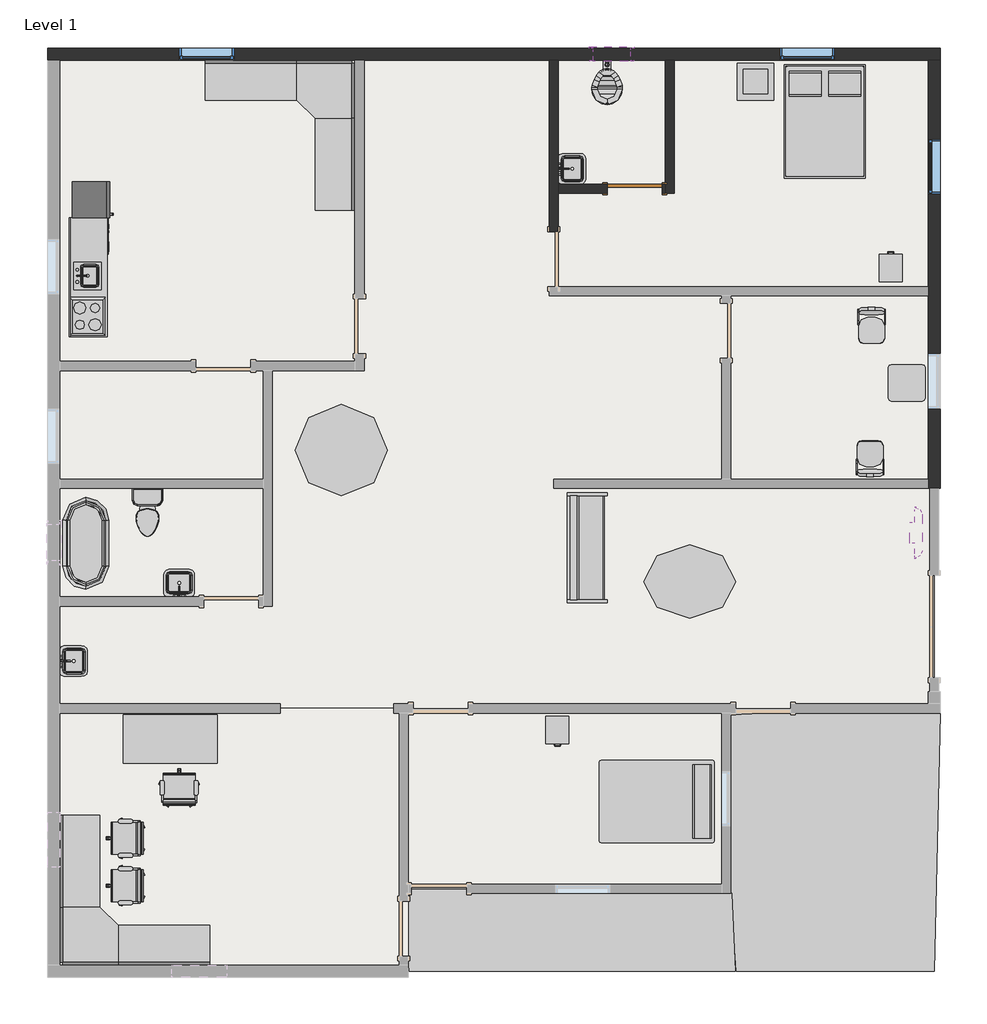
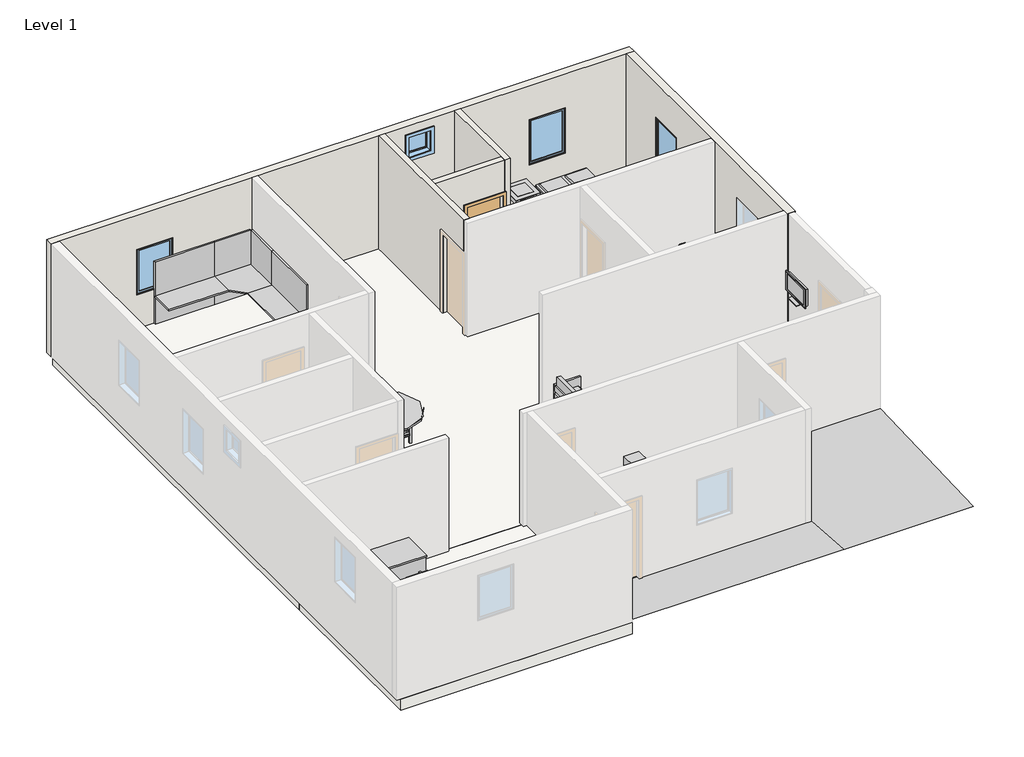
# One storey, part 2 of 2: 19 furniture elements, 7 flow terminals, 6 proxies, 5 walls, 4 windows, 3 slabs, 1 door.
"""IFC4 building model written with IfcOpenShell, lengths in millimetres."""

from ifc_helpers import new_model, si_unit, frame, origin, place, context, project, spatial, polyline, outline, extrude, faceted_brep, triangles, transform, mapped, element, save
from components import proxy_a6faaae8, proxy_45b28599, kitchenette_medium_kitchenette_medium_844211aa, proxy_c523a7b7, door_16372e1c, flow_terminal_871c2e40, flow_terminal_62a433f7, flow_terminal_bd37145e, toilet_domestic_3d_toilet_domestic_3d_f7549cf7, toilet_domestic_3d_toilet_domestic_3d_183bbd19, flow_terminal_b374fae2, furniture_c8abb964, furniture_0253826f, furniture_bb55ed6b, furniture_552c1472, chair_task_arms_chair_task_arms_fa5a08ef, furniture_c6510c7c, furniture_013ab306, furniture_3d1d9cbc, furniture_a4ffab56, furniture_56245f3a, furniture_b5c51a22, furniture_bbcc68ce, furniture_743965d2, furniture_bcf351fa, furniture_45e3acac, window_e2841890, window_e41d21a6

model = new_model("IFC4")

# Units and contexts
model_context = context("Model", 3, world=origin())
ifc_project = project(units=[si_unit("LENGTHUNIT", "METRE", prefix="MILLI")], contexts=[model_context])

# Site, building, storey
site = spatial("IfcSite", under=ifc_project)
building = spatial("IfcBuilding", under=site)
storey = spatial("IfcBuildingStorey", under=building, Name="Level 1", Elevation=0.0)

# Proxies
placement = place(None, origin())
element("IfcBuildingElementProxy", 1, Name="Building Element Proxy", at=placement, inside=storey, context=model_context, shape_type="Tessellation", body=[
    triangles([(-9324.3738739, -3265.5495117, 0.0), (-9375.1736801, -4560.9495117, 0.0), (-4015.773777, -3367.1497055, 0.0), (-3955.7570915, -4662.5497055, 0.0), (-9375.1736801, -3770.3762558, 0.0), (-9349.7740677, -3612.3260193, 0.0), (-9412.73069, -3494.1495117, 0.0), (-9416.536853, -3494.1495117, 0.0), (-9427.1478333, -3494.1495117, 0.0), (-9437.6187057, -3847.712233, 0.0), (-9375.1736801, -4662.5497055, 0.0), (-8521.0984863, -3265.5495117, 0.0), (-9434.5572647, -3550.4170074, 0.0), (-9438.7442184, -3503.4963249, 0.0)], [[7, 13, 6], [10, 5, 13], [10, 13, 14], [14, 9, 1], [9, 14, 8], [8, 7, 1], [8, 14, 13], [13, 7, 8], [9, 8, 1], [10, 11, 2], [5, 2, 12], [12, 11, 4], [2, 11, 12], [2, 5, 10], [1, 7, 6], [1, 6, 12], [12, 6, 5], [4, 3, 12], [6, 13, 5]], closed=False),
])
element("IfcBuildingElementProxy", 2, Name="Building Element Proxy", at=placement, inside=storey, context=model_context, shape_type="Tessellation", body=[
    triangles([(-4028.4738739, -395.3495965, 0.0), (-548.6738133, -369.9496207, 0.0), (-650.2738255, -4662.5497055, 0.0), (-3938.4880875, -4662.5497055, 0.0), (-4028.4738739, -3367.1497055, 0.0), (-3495.0738739, -369.9496207, 0.0)], [[6, 1, 5], [3, 5, 4], [5, 2, 6], [2, 5, 3]], closed=False),
])
proxy_shape = proxy_a6faaae8(model_context)
element("IfcBuildingElementProxy", 3, Name="Cook Top-4 Unit2 : 22\" x 20\"", ObjectType="Cook Top-4 Unit2 : 22\" x 20\"", at=placement, inside=storey, context=model_context, shape_type="MappedRepresentation", body=[
    mapped(proxy_shape, transform((-14721.8737976, 6221.350395, 0.0), x_axis=(0.0, 1.0000000000000002, 0.0), y_axis=(-1.0000000000000002, 0.0, 0.0), z_axis=(0.0, 0.0, 1.0))),
])
proxy_2_shape = proxy_45b28599(model_context)
element("IfcBuildingElementProxy", 4, Name="Dishwasher : 24\" x 24\" x 34\"", ObjectType="Dishwasher : 24\" x 24\" x 34\"", at=placement, inside=storey, context=model_context, shape_type="MappedRepresentation", body=[
    mapped(proxy_2_shape, transform((-14430.0242329, 7172.5329265, 0.0), x_axis=(0.0, 1.0000000000000002, 0.0), y_axis=(-1.0000000000000002, 0.0, 0.0), z_axis=(0.0, 0.0, 1.0))),
])
kitchenette_medium_kitchenette_medium_shape = kitchenette_medium_kitchenette_medium_844211aa(model_context)
element("IfcBuildingElementProxy", 5, Name="Kitchenette - Medium : Kitchenette - Medium", ObjectType="Kitchenette - Medium : Kitchenette - Medium", at=placement, inside=storey, context=model_context, shape_type="MappedRepresentation", body=[
    mapped(kitchenette_medium_kitchenette_medium_shape, transform((-15026.6737976, 6545.5126901, 0.0), x_axis=(0.0, 1.0000000000000002, 0.0), y_axis=(-1.0000000000000002, 0.0, 0.0), z_axis=(0.0, 0.0, 1.0))),
])
proxy_3_shape = proxy_c523a7b7(model_context)
element("IfcBuildingElementProxy", 6, Name="Refrigerator : 24\" x 25\" LH", ObjectType="Refrigerator : 24\" x 25\" LH", at=placement, inside=storey, context=model_context, shape_type="MappedRepresentation", body=[
    mapped(proxy_3_shape, transform((-14676.2248262, 8158.100395, 0.0), x_axis=(0.0, 1.0000000000000002, 0.0), y_axis=(-1.0000000000000002, 0.0, 0.0), z_axis=(0.0, 0.0, 1.0))),
])

# Door
door_shape = door_16372e1c(model_context)
element("IfcDoor", 7, ObjectType="Single-Flush : 36\" x 84\"", at=placement, inside=storey, context=model_context, shape_type="MappedRepresentation", body=[
    mapped(door_shape, transform((-5628.6737976, 8342.250395, 0.0), x_axis=(1.0, 0.0, 0.0), y_axis=(0.0, 1.0, 0.0), z_axis=(0.0, 0.0, 1.0))),
])

# Flow terminals
flow_terminal_shape = flow_terminal_871c2e40(model_context)
element("IfcFlowTerminal", 8, ObjectType="Sink Kitchen-Island : 18\" x 18\"", at=placement, inside=storey, context=model_context, shape_type="MappedRepresentation", body=[
    mapped(flow_terminal_shape, transform((-14719.5283965, 6878.7611544, -14.4), x_axis=(0.0, 1.0000000000000002, 0.0), y_axis=(-1.0000000000000002, 0.0, 0.0), z_axis=(0.0, 0.0, 1.0))),
])
flow_terminal_2_shape = flow_terminal_62a433f7(model_context)
element("IfcFlowTerminal", 9, ObjectType="Sink Vanity-Square : 20\" x 18\"", at=placement, inside=storey, context=model_context, shape_type="MappedRepresentation", body=[
    mapped(flow_terminal_2_shape, transform((-13182.1845571, 1740.5957961, 0.0), x_axis=(-1.0000000000000004, 0.0, 0.0), y_axis=(0.0, -1.0000000000000004, 0.0), z_axis=(0.0, 0.0, 1.0))),
])
element("IfcFlowTerminal", 10, ObjectType="Sink Vanity-Square : 20\" x 18\"", at=placement, inside=storey, context=model_context, shape_type="MappedRepresentation", body=[
    mapped(flow_terminal_2_shape, transform((-14998.9283965, 477.9611544, 0.0), x_axis=(0.0, 1.0000000000000002, 0.0), y_axis=(-1.0000000000000002, 0.0, 0.0), z_axis=(0.0, 0.0, 1.0))),
])
element("IfcFlowTerminal", 11, ObjectType="Sink Vanity-Square : 20\" x 18\"", at=placement, inside=storey, context=model_context, shape_type="MappedRepresentation", body=[
    mapped(flow_terminal_2_shape, transform((-6718.5283965, 8656.7611544, 0.0), x_axis=(0.0, 1.0, 0.0), y_axis=(-1.0, 0.0, 0.0), z_axis=(0.0, 0.0, 1.0))),
])
flow_terminal_3_shape = flow_terminal_bd37145e(model_context)
element("IfcFlowTerminal", 12, ObjectType="Toilet-Commercial-Wall-3D : 15\" Seat Height", at=placement, inside=storey, context=model_context, shape_type="MappedRepresentation", body=[
    mapped(flow_terminal_3_shape, transform((-5680.9706438, 10577.450395, 0.0), x_axis=(-1.0, 0.0, 0.0), y_axis=(0.0, -1.0, 0.0), z_axis=(0.0, 0.0, 1.0))),
])
toilet_domestic_3d_toilet_domestic_3d_shape = toilet_domestic_3d_toilet_domestic_3d_f7549cf7(model_context)
toilet_domestic_3d_toilet_domestic_3d_2_shape = toilet_domestic_3d_toilet_domestic_3d_183bbd19(model_context)
element("IfcFlowTerminal", 13, ObjectType="Toilet-Domestic-3D : Toilet-Domestic-3D", at=placement, inside=storey, context=model_context, shape_type="MappedRepresentation", body=[
    mapped(toilet_domestic_3d_toilet_domestic_3d_shape, transform((-13724.1724957, 2869.1543677, 0.0), x_axis=(1.0, 0.0, 0.0), y_axis=(0.0, 1.0, 0.0), z_axis=(0.0, 0.0, 1.0))),
    mapped(toilet_domestic_3d_toilet_domestic_3d_2_shape, transform((-13724.1724957, 2869.1543677, 0.0), x_axis=(1.0, 0.0, 0.0), y_axis=(0.0, 1.0, 0.0), z_axis=(0.0, 0.0, 1.0))),
])
flow_terminal_4_shape = flow_terminal_b374fae2(model_context)
element("IfcFlowTerminal", 14, ObjectType="Tub-Free Standing-3D : 30\" x 60\"", at=placement, inside=storey, context=model_context, shape_type="MappedRepresentation", body=[
    mapped(flow_terminal_4_shape, transform((-14747.2737976, 2449.450395, 0.0), x_axis=(1.0, 0.0, 0.0), y_axis=(0.0, 1.0, 0.0), z_axis=(0.0, 0.0, 1.0))),
])

# Furniture
furniture_shape = furniture_c8abb964(model_context)
element("IfcFurniture", 15, ObjectType="Bed-Box : Double 53\" x 74\"", at=placement, inside=storey, context=model_context, shape_type="MappedRepresentation", body=[
    mapped(furniture_shape, transform((-2805.5262567, 9694.2799032, 0.0), x_axis=(1.0, 0.0, 0.0), y_axis=(0.0, 1.0, 0.0), z_axis=(0.0, 0.0, 1.0))),
])
furniture_2_shape = furniture_0253826f(model_context)
element("IfcFurniture", 16, ObjectType="Bed-Standard : Double 54\" x 75\"", at=placement, inside=storey, context=model_context, shape_type="MappedRepresentation", body=[
    mapped(furniture_2_shape, transform((-5214.7787157, -1571.6610804, 0.0), x_axis=(0.0, -1.0000000000000002, 0.0), y_axis=(1.0000000000000002, 0.0, 0.0), z_axis=(0.0, 0.0, 1.0))),
])
furniture_3_shape = furniture_bb55ed6b(model_context)
element("IfcFurniture", 17, ObjectType="Cabinet-File 2 Drawer : 15\" x 18\"", at=placement, inside=storey, context=model_context, shape_type="MappedRepresentation", body=[
    mapped(furniture_3_shape, transform((-1502.0702447, 6879.3160949, 0.0), x_axis=(-1.0000000000000002, 0.0, 0.0), y_axis=(0.0, -1.0000000000000002, 0.0), z_axis=(0.0, 0.0, 1.0))),
])
furniture_4_shape = furniture_552c1472(model_context)
element("IfcFurniture", 18, ObjectType="Cabinet-File 3 Drawer : 15\" x 18\"", at=placement, inside=storey, context=model_context, shape_type="MappedRepresentation", body=[
    mapped(furniture_4_shape, transform((-6783.4773506, -507.2153049, 0.0), x_axis=(1.0, 0.0, 0.0), y_axis=(0.0, 1.0, 0.0), z_axis=(0.0, 0.0, 1.0))),
])
chair_task_arms_chair_task_arms_shape = chair_task_arms_chair_task_arms_fa5a08ef(model_context)
element("IfcFurniture", 19, ObjectType="Chair-Task Arms : Chair-Task Arms", at=placement, inside=storey, context=model_context, shape_type="MappedRepresentation", body=[
    mapped(chair_task_arms_chair_task_arms_shape, transform((-13338.8646173, -1658.8955066, 0.0), x_axis=(1.0000000000000007, 0.0, 0.0), y_axis=(0.0, 1.0000000000000007, 0.0), z_axis=(0.0, 0.0, 1.0))),
])
element("IfcFurniture", 20, ObjectType="Chair-Task Arms : Chair-Task Arms", at=placement, inside=storey, context=model_context, shape_type="MappedRepresentation", body=[
    mapped(chair_task_arms_chair_task_arms_shape, transform((-14042.527896, -2593.7404247, 0.0), x_axis=(0.0, 1.0, 0.0), y_axis=(-1.0, 0.0, 0.0), z_axis=(0.0, 0.0, 1.0))),
])
element("IfcFurniture", 21, ObjectType="Chair-Task Arms : Chair-Task Arms", at=placement, inside=storey, context=model_context, shape_type="MappedRepresentation", body=[
    mapped(chair_task_arms_chair_task_arms_shape, transform((-14042.527896, -3381.1404247, 0.0), x_axis=(0.0, 1.0, 0.0), y_axis=(-1.0, 0.0, 0.0), z_axis=(0.0, 0.0, 1.0))),
])
furniture_5_shape = furniture_c6510c7c(model_context)
element("IfcFurniture", 22, ObjectType="Counter Top w Sink Hole : 24\" Depth", at=placement, inside=storey, context=model_context, shape_type="MappedRepresentation", body=[
    mapped(furniture_5_shape, transform((-15026.6737976, 7078.9126901, -14.4), x_axis=(0.0, 1.0000000000000002, 0.0), y_axis=(-1.0000000000000002, 0.0, 0.0), z_axis=(0.0, 0.0, 1.0))),
])
furniture_6_shape = furniture_013ab306(model_context)
element("IfcFurniture", 23, ObjectType="Desk : 60\" x 30\" Student", at=placement, inside=storey, context=model_context, shape_type="MappedRepresentation", body=[
    mapped(furniture_6_shape, transform((-12581.619432, -420.749605, 0.0), x_axis=(-1.0000000000000002, 0.0, 0.0), y_axis=(0.0, -1.0000000000000002, 0.0), z_axis=(0.0, 0.0, 1.0))),
])
furniture_7_shape = furniture_3d1d9cbc(model_context)
element("IfcFurniture", 24, ObjectType="Seating-Auditorium : 18\" x 24\" x 30\"", at=placement, inside=storey, context=model_context, shape_type="MappedRepresentation", body=[
    mapped(furniture_7_shape, transform((-1530.9459288, 6271.5258048, 0.0), x_axis=(-1.0000000000000004, 0.0, 0.0), y_axis=(0.0, -1.0000000000000004, 0.0), z_axis=(0.0, 0.0, 1.0))),
])
element("IfcFurniture", 25, ObjectType="Seating-Auditorium : 18\" x 24\" x 30\"", at=placement, inside=storey, context=model_context, shape_type="MappedRepresentation", body=[
    mapped(furniture_7_shape, transform((-1877.8016665, 3656.5749852, 0.0), x_axis=(1.0, 0.0, 0.0), y_axis=(0.0, 1.0, 0.0), z_axis=(0.0, 0.0, 1.0))),
])
furniture_8_shape = furniture_a4ffab56(model_context)
element("IfcFurniture", 26, ObjectType="Sofa : 72\"", at=placement, inside=storey, context=model_context, shape_type="MappedRepresentation", body=[
    mapped(furniture_8_shape, transform((-6269.9196993, 2302.8799032, 0.0), x_axis=(0.0, 1.0000000000000002, 0.0), y_axis=(-1.0000000000000002, 0.0, 0.0), z_axis=(0.0, 0.0, 1.0))),
])
furniture_9_shape = furniture_56245f3a(model_context)
element("IfcFurniture", 27, ObjectType="TV - Flat Screen : 32\"", at=placement, inside=storey, context=model_context, shape_type="MappedRepresentation", body=[
    mapped(furniture_9_shape, transform((-907.1288655, 2623.3058809, 1219.2), x_axis=(0.0, -1.0000000000000007, 0.0), y_axis=(1.0000000000000007, 0.0, 0.0), z_axis=(0.0, 0.0, 1.0))),
])
furniture_10_shape = furniture_b5c51a22(model_context)
element("IfcFurniture", 28, ObjectType="Table-Coffee : 24\" x 24\" x 24\"", at=placement, inside=storey, context=model_context, shape_type="MappedRepresentation", body=[
    mapped(furniture_10_shape, transform((-3640.3395643, 10025.0393172, 0.0), x_axis=(1.0, 0.0, 0.0), y_axis=(0.0, 1.0, 0.0), z_axis=(0.0, 0.0, 1.0))),
])
furniture_11_shape = furniture_bbcc68ce(model_context)
element("IfcFurniture", 29, ObjectType="Table-Dining Round w Chairs : 60\" Diameter", at=placement, inside=storey, context=model_context, shape_type="MappedRepresentation", body=[
    mapped(furniture_11_shape, transform((-10609.1557649, 4183.7290835, 0.0), x_axis=(1.0, 0.0, 0.0), y_axis=(0.0, 1.0, 0.0), z_axis=(0.0, 0.0, 1.0))),
])
furniture_12_shape = furniture_743965d2(model_context)
element("IfcFurniture", 30, ObjectType="Table-Ellipse : 60\" x 48\"", at=placement, inside=storey, context=model_context, shape_type="MappedRepresentation", body=[
    mapped(furniture_12_shape, transform((-4714.2737976, 1814.450395, 0.0), x_axis=(1.0, 0.0, 0.0), y_axis=(0.0, 1.0, 0.0), z_axis=(0.0, 0.0, 1.0))),
])
furniture_13_shape = furniture_bcf351fa(model_context)
element("IfcFurniture", 31, ObjectType="Table-End : 24\" x 24\"", at=placement, inside=storey, context=model_context, shape_type="MappedRepresentation", body=[
    mapped(furniture_13_shape, transform((-1416.0074279, 4964.050395, 0.0), x_axis=(1.0, 0.0, 0.0), y_axis=(0.0, 1.0, 0.0), z_axis=(0.0, 0.0, 1.0))),
])
furniture_14_shape = furniture_45e3acac(model_context)
element("IfcFurniture", 32, ObjectType="Work Station Cubicle : 96\" x 96\"", at=placement, inside=storey, context=model_context, shape_type="MappedRepresentation", body=[
    mapped(furniture_14_shape, transform((-9781.85079, 10344.1186428, 0.0), x_axis=(0.0, -1.0000000000000004, 0.0), y_axis=(1.0000000000000004, 0.0, 0.0), z_axis=(0.0, 0.0, 1.0))),
])
element("IfcFurniture", 33, ObjectType="Work Station Cubicle : 96\" x 96\"", at=placement, inside=storey, context=model_context, shape_type="MappedRepresentation", body=[
    mapped(furniture_14_shape, transform((-15674.0968053, -4429.2178528, 0.0), x_axis=(0.0, 1.0000000000000002, 0.0), y_axis=(-1.0000000000000002, 0.0, 0.0), z_axis=(0.0, 0.0, 1.0))),
])

# Slabs
element("IfcSlab", 34, ObjectType="Generic - 12\"", at=placement, inside=storey, context=model_context, shape_type="SweptSolid", body=[
    extrude(outline(polyline([(-650.2737976, 10577.450395), (-650.2737976, -293.749605), (-15280.6737976, -293.749605), (-15280.6737976, 10577.450395), (-650.2737976, 10577.450395)])), frame((0.0, 0.0, -304.8), z_axis=(0.0, 0.0, 1.0), x_axis=(1.0, 0.0, 0.0)), (0.0, 0.0, 1.0), 304.8),
])
element("IfcSlab", 35, ObjectType="Generic - 12\"", at=placement, inside=storey, context=model_context, shape_type="SweptSolid", body=[
    extrude(outline(polyline([(-9387.8737976, -293.749605), (-9387.8737976, -4764.149605), (-15280.6737976, -4764.149605), (-15280.6737976, -293.749605), (-9387.8737976, -293.749605)])), frame((0.0, 0.0, -304.8), z_axis=(0.0, 0.0, 1.0), x_axis=(1.0, 0.0, 0.0)), (0.0, 0.0, 1.0), 304.8),
])
element("IfcSlab", 36, ObjectType="Generic - 12\"", at=placement, inside=storey, context=model_context, shape_type="SweptSolid", body=[
    extrude(outline(polyline([(-4104.6737976, -369.949605), (-4104.6737976, -3290.949605), (-9387.8737976, -3290.949605), (-9387.8737976, -369.949605), (-4104.6737976, -369.949605)])), frame((0.0, 0.0, -304.8), z_axis=(0.0, 0.0, 1.0), x_axis=(1.0, 0.0, 0.0)), (0.0, 0.0, 1.0), 304.8),
])

# Walls
element("IfcWall", 37, ObjectType="Generic - 8\"", at=placement, inside=storey, context=model_context, shape_type="Brep", body=[
    faceted_brep([(-15382.2737976, 10475.850395, 0.0), (-15179.0737976, 10475.850395, 0.0), (-10276.8737976, 10475.850395, 0.0), (-10124.4737976, 10475.850395, 0.0), (-7051.0737976, 10475.850395, 0.0), (-6898.6737976, 10475.850395, 0.0), (-5120.6737976, 10475.850395, 0.0), (-4968.2737976, 10475.850395, 0.0), (-751.8737976, 10475.850395, 0.0), (-548.6737976, 10475.850395, 0.0), (-548.6737976, 10475.850395, 3048.0), (-751.8737976, 10475.850395, 3048.0), (-4968.2737976, 10475.850395, 3048.0), (-5120.6737976, 10475.850395, 3048.0), (-6898.6737976, 10475.850395, 3048.0), (-7051.0737976, 10475.850395, 3048.0), (-10124.4737976, 10475.850395, 3048.0), (-10276.8737976, 10475.850395, 3048.0), (-15179.0737976, 10475.850395, 3048.0), (-15382.2737976, 10475.850395, 3048.0), (-13197.8737976, 10475.850395, 2133.6), (-12283.4737976, 10475.850395, 2133.6), (-12283.4737976, 10475.850395, 914.4), (-13197.8737976, 10475.850395, 914.4), (-3215.6737976, 10475.850395, 2133.6), (-2301.2737976, 10475.850395, 2133.6), (-2301.2737976, 10475.850395, 914.4), (-3215.6737976, 10475.850395, 914.4), (-5704.8737976, 10475.850395, 2768.6), (-5704.8737976, 10475.850395, 2159.0), (-6314.4737976, 10475.850395, 2159.0), (-6314.4737976, 10475.850395, 2768.6), (-15382.2737976, 10679.050395, 0.0), (-15382.2737976, 10679.050395, 3048.0), (-548.6737976, 10679.050395, 3048.0), (-548.6737976, 10679.050395, 0.0), (-13197.8737976, 10679.050395, 2133.6), (-13197.8737976, 10679.050395, 914.4), (-12283.4737976, 10679.050395, 914.4), (-12283.4737976, 10679.050395, 2133.6), (-3215.6737976, 10679.050395, 2133.6), (-3215.6737976, 10679.050395, 914.4), (-2301.2737976, 10679.050395, 914.4), (-2301.2737976, 10679.050395, 2133.6), (-5704.8737976, 10679.050395, 2768.6), (-6314.4737976, 10679.050395, 2768.6), (-6314.4737976, 10679.050395, 2159.0), (-5704.8737976, 10679.050395, 2159.0)], [[[0, 1, 2, 3, 4, 5, 6, 7, 8, 9, 10, 11, 12, 13, 14, 15, 16, 17, 18, 19], [20, 21, 22, 23], [24, 25, 26, 27], [28, 29, 30, 31]], [[32, 33, 34, 35], [36, 37, 38, 39], [40, 41, 42, 43], [44, 45, 46, 47]], [[9, 8, 7, 6, 5, 4, 3, 2, 1, 0, 32, 35]], [[19, 18, 17, 16, 15, 14, 13, 12, 11, 10, 34, 33]], [[10, 9, 35, 34]], [[0, 19, 33, 32]], [[37, 36, 20, 23]], [[38, 37, 23, 22]], [[39, 38, 22, 21]], [[36, 39, 21, 20]], [[41, 40, 24, 27]], [[42, 41, 27, 26]], [[43, 42, 26, 25]], [[40, 43, 25, 24]], [[29, 28, 44, 47]], [[30, 29, 47, 46]], [[31, 30, 46, 45]], [[28, 31, 45, 44]]]),
])
element("IfcWall", 38, ObjectType="Generic - 8\"", at=placement, inside=storey, context=model_context, shape_type="Brep", body=[
    faceted_brep([(-751.8737976, 10475.850395, 0.0), (-751.8737976, 6716.650395, 0.0), (-751.8737976, 6564.250395, 0.0), (-751.8737976, 3516.250395, 0.0), (-751.8737976, 3363.850395, 0.0), (-751.8737976, 3363.850395, 3048.0), (-751.8737976, 3516.250395, 3048.0), (-751.8737976, 6564.250395, 3048.0), (-751.8737976, 6716.650395, 3048.0), (-751.8737976, 10475.850395, 3048.0), (-751.8737976, 4684.650395, 2133.6), (-751.8737976, 4684.650395, 914.4), (-751.8737976, 5599.050395, 914.4), (-751.8737976, 5599.050395, 2133.6), (-751.8737976, 9167.750395, 2133.6), (-751.8737976, 8253.350395, 2133.6), (-751.8737976, 8253.350395, 914.4), (-751.8737976, 9167.750395, 914.4), (-548.6737976, 10475.850395, 0.0), (-548.6737976, 10475.850395, 3048.0), (-548.6737976, 3363.850395, 3048.0), (-548.6737976, 3363.850395, 0.0), (-548.6737976, 4684.650395, 2133.6), (-548.6737976, 5599.050395, 2133.6), (-548.6737976, 5599.050395, 914.4), (-548.6737976, 4684.650395, 914.4), (-548.6737976, 9167.750395, 2133.6), (-548.6737976, 9167.750395, 914.4), (-548.6737976, 8253.350395, 914.4), (-548.6737976, 8253.350395, 2133.6), (-574.0737976, 3363.850395, 0.0), (-726.4737976, 3363.850395, 0.0), (-726.4737976, 3363.850395, 3048.0), (-574.0737976, 3363.850395, 3048.0)], [[[0, 1, 2, 3, 4, 5, 6, 7, 8, 9], [10, 11, 12, 13], [14, 15, 16, 17]], [[18, 19, 20, 21], [22, 23, 24, 25], [26, 27, 28, 29]], [[4, 3, 2, 1, 0, 18, 21, 30, 31]], [[9, 8, 7, 6, 5, 32, 33, 20, 19]], [[0, 9, 19, 18]], [[11, 10, 22, 25]], [[12, 11, 25, 24]], [[13, 12, 24, 23]], [[10, 13, 23, 22]], [[27, 26, 14, 17]], [[28, 27, 17, 16]], [[29, 28, 16, 15]], [[26, 29, 15, 14]], [[5, 4, 31, 30, 21, 20, 33, 32]]]),
])
element("IfcWall", 39, ObjectType="INNER WALL 6\"", at=placement, inside=storey, context=model_context, shape_type="Brep", body=[
    faceted_brep([(-6898.6737976, 10475.850395, 3048.0), (-6898.6737976, 8418.450395, 3048.0), (-6898.6737976, 8266.050395, 3048.0), (-6898.6737976, 6716.650395, 3048.0), (-6898.6737976, 6716.650395, 2133.6), (-6898.6737976, 7631.050395, 2133.6), (-6898.6737976, 7631.050395, 0.0), (-6898.6737976, 8266.050395, 0.0), (-6898.6737976, 8418.450395, 0.0), (-6898.6737976, 10475.850395, 0.0), (-7051.0737976, 6716.650395, 3048.0), (-7051.0737976, 10475.850395, 3048.0), (-7051.0737976, 10475.850395, 0.0), (-7051.0737976, 7631.050395, 0.0), (-7051.0737976, 7631.050395, 2133.6), (-7051.0737976, 6716.650395, 2133.6)], [[[0, 1, 2, 3, 4, 5, 6, 7, 8, 9]], [[10, 11, 12, 13, 14, 15]], [[12, 9, 8, 7, 6, 13]], [[3, 2, 1, 0, 11, 10]], [[3, 10, 15, 4]], [[0, 9, 12, 11]], [[14, 5, 4, 15]], [[5, 14, 13, 6]]]),
])
element("IfcWall", 40, ObjectType="INNER WALL 6\"", at=placement, inside=storey, context=model_context, shape_type="Brep", body=[
    faceted_brep([(-5120.6737976, 10475.850395, 0.0), (-5120.6737976, 8418.450395, 0.0), (-5120.6737976, 8266.050395, 0.0), (-5120.6737976, 8266.050395, 3048.0), (-5120.6737976, 8418.450395, 3048.0), (-5120.6737976, 10475.850395, 3048.0), (-4968.2737976, 10475.850395, 0.0), (-4968.2737976, 10475.850395, 3048.0), (-4968.2737976, 8266.050395, 3048.0), (-4968.2737976, 8266.050395, 0.0)], [[[0, 1, 2, 3, 4, 5]], [[6, 7, 8, 9]], [[2, 1, 0, 6, 9]], [[5, 4, 3, 8, 7]], [[0, 5, 7, 6]], [[3, 2, 9, 8]]]),
])
element("IfcWall", 41, ObjectType="INNER WALL 6\"", at=placement, inside=storey, context=model_context, shape_type="SweptSolid", body=[
    extrude(outline(polyline([(2133.6, -5171.4737976), (0.0, -5171.4737976), (0.0, -5120.6737976), (3048.0, -5120.6737976), (3048.0, -6898.6737976), (0.0, -6898.6737976), (0.0, -6085.8737976), (2133.6, -6085.8737976), (2133.6, -5171.4737976)])), frame((0.0, 8266.050395, 0.0), z_axis=(0.0, 1.0, 0.0), x_axis=(0.0, 0.0, 1.0)), (0.0, 0.0, 1.0), 152.4),
])

# Windows
window_shape = window_e2841890(model_context)
element("IfcWindow", 42, ObjectType="Fixed : 36\" x 48\"", at=placement, inside=storey, context=model_context, shape_type="MappedRepresentation", body=[
    mapped(window_shape, transform((-12778.7737976, 10577.450395, 0.0), x_axis=(-1.0, 0.0, 0.0), y_axis=(0.0, -1.0, 0.0), z_axis=(0.0, 0.0, 1.0))),
])
element("IfcWindow", 43, ObjectType="Fixed : 36\" x 48\"", at=placement, inside=storey, context=model_context, shape_type="MappedRepresentation", body=[
    mapped(window_shape, transform((-650.2737976, 8748.650395, 0.0), x_axis=(0.0, 1.0, 0.0), y_axis=(-1.0, 0.0, 0.0), z_axis=(0.0, 0.0, 1.0))),
])
element("IfcWindow", 44, ObjectType="Fixed : 36\" x 48\"", at=placement, inside=storey, context=model_context, shape_type="MappedRepresentation", body=[
    mapped(window_shape, transform((-2796.5737976, 10577.450395, 0.0), x_axis=(-1.0, 0.0, 0.0), y_axis=(0.0, -1.0, 0.0), z_axis=(0.0, 0.0, 1.0))),
])
window_2_shape = window_e41d21a6(model_context)
element("IfcWindow", 45, ObjectType="Transom with Trim : 24\" x 24\"", at=placement, inside=storey, context=model_context, shape_type="MappedRepresentation", body=[
    mapped(window_2_shape, transform((-5971.5737976, 10577.450395, 0.0), x_axis=(1.0, 0.0, 0.0), y_axis=(0.0, 1.0, 0.0), z_axis=(0.0, 0.0, 1.0))),
])

save(model, "model.ifc")

# Revit data of these elements
# Type "Cook Top-4 Unit2 : 22\" x 20\""
#   Depth = 1' - 8"
#   Width = 1' - 10"
#   Burner Material = Steel, Chrome Plated
#   Cooktop Material = Steel, Polished
#   Default Elevation = 0
#   Assembly Code = ""
# Type "Dishwasher : 24\" x 24\" x 34\""
#   Label = "DW"
#   Assembly Code = "E1090400"
#   Depth = 2' - 0"
#   Height = 2' - 10"
#   Width = 2' - 0"
#   Dishwasher Material = Steel, Paint Finish, Ivory, Glossy
#   Panel Face Material = Plastic, Opaque Black
#   Default Elevation = 0
# Type "Kitchenette - Medium : Kitchenette - Medium"
#   Assembly Code = "E1090400"
#   Counter Length = 6' - 6"
#   Cabinet Width = 4' - 6"
#   Cabinet Height = 2' - 10 1/2"
#   Cabinet Depth = 2' - 0"
#   Toe Depth = 0' - 3"
#   Toe Height = 0' - 3 1/2"
#   Cabinet Material = Cabinets
#   Door/Drawer Material = Cabinets
#   Handle Material = Cabinets - Handles
#   Default Elevation = 0
# Type "Refrigerator : 24\" x 25\" LH"
#   Label = "REF."
#   Assembly Code = "E1090400"
#   Depth = 2' - 0 3/4"
#   Handle = 0' - 1 1/2"
#   Height = 5' - 3 1/2"
#   Rear Clearance = 0' - 2"
#   Top Door Height = 1' - 8"
#   Width = 1' - 11 1/2"
#   Material = Steel, Paint Finish, Ivory, Glossy
#   Default Elevation = 0
# Type "Single-Flush : 36\" x 84\""
#   Type Mark = "1"
#   Construction Type Id = "MDOOR"
#   Assembly Code = "C1020"
#   Analytic Construction = "Metal"
#   Thickness = 0' - 2"
#   Heat Transfer Coefficient (U) = 0.651978 BTU/(h·ft²·°F)
#   Height = 7' - 0"
#   Trim Projection Ext = 0' - 1"
#   Trim Projection Int = 0' - 1"
#   Trim Width = 0' - 3"
#   Width = 3' - 0"
#   Define Thermal Properties by = 1
#   Door Material = Door - Panel
#   Frame Material = Door - Frame
#   Visual Light Transmittance = 0
#   Solar Heat Gain Coefficient = 0
#   Function = (empty or 0)
#   Wall Closure = (empty or 0)
# Type "Sink Kitchen-Island : 18\" x 18\""
#   Assembly Code = "D2010410"
#   Counter Height = 3' - 0"
#   Depth = 1' - 6"
#   Width = 1' - 6"
#   Faucet Material = Steel, Polished
#   Sink Material = Steel, Polished
#   Default Elevation = 0
# Type "Sink Vanity-Square : 20\" x 18\""
#   Assembly Code = "D2010400"
#   Counter Height = 2' - 7"
#   Depth = 1' - 6"
#   Width = 1' - 8"
#   Basin Material = Porcelain, Linen
#   Faucet Material = Steel, Polished
#   Default Elevation = 0
# Type "Toilet-Commercial-Wall-3D : 15\" Seat Height"
#   Assembly Code = "D2010110"
#   Mounting Height = 1' - 3"
#   Piping Material = Steel, Polished
#   Toilet - Bowl Material = Porcelain, Ivory
#   Toilet - Seat Material = Laminate, Ivory, Matte
#   Default Elevation = 0
# Type "Toilet-Domestic-3D : Toilet-Domestic-3D"
#   Assembly Code = "D2010110"
#   Toilet - Bowl/Basin Material = Porcelain, Linen
#   Toilet - Seat Material = Laminate, Linen, Matte
#   Default Elevation = 0
# Type "Tub-Free Standing-3D : 30\" x 60\""
#   Assembly Code = "D2010110"
#   Height = 1' - 6"
#   Length = 5' - 0"
#   Width = 2' - 6"
#   Tub Material = Porcelain, Ivory
#   Default Elevation = 0
# Type "Bed-Box : Double 53\" x 74\""
#   Assembly Code = "E2020200"
#   Length = 6' - 2"
#   Width = 4' - 5"
#   Frame Material = Birch
#   Mattress Material = Linen, White
#   Default Elevation = 0
# Type "Bed-Standard : Double 54\" x 75\""
#   Assembly Code = "E2020200"
#   Length = 6' - 3"
#   Width = 4' - 6"
#   Leg Material = Steel, Chrome Plated
#   Mattress Material = Linen, White
#   Default Elevation = 0
# Type "Cabinet-File 2 Drawer : 15\" x 18\""
#   Assembly Code = "E2020200"
#   Depth = 1' - 6"
#   Height = 2' - 5"
#   Width = 1' - 3"
#   Cabinet Material = Steel, Paint Finish, Ivory, Glossy
#   Handle Material = Steel, Chrome Plated
#   Default Elevation = 0
# Type "Cabinet-File 3 Drawer : 15\" x 18\""
#   Assembly Code = "E2020200"
#   Depth = 1' - 6"
#   Height = 3' - 5"
#   Width = 1' - 3"
#   Cabinet Material = Steel, Paint Finish, Ivory, Glossy
#   Handle Material = Steel, Chrome Plated
#   Default Elevation = 0
# Type "Chair-Task Arms : Chair-Task Arms"
#   Assembly Code = "E2020200"
#   Base Material = Plastic, Opaque Black
#   Caster Material = Plastic, Opaque Black
#   Seat/Back Material = Textile - Slate Blue
#   Default Elevation = 0
# Type "Counter Top w Sink Hole : 24\" Depth"
#   Assembly Code = "C1030400"
#   Counter Thickness = 0' - 1 1/2"
#   Depth = 2' - 1"
#   Height = 3' - 0"
#   Length [instance default] = 8' - 0"
#   Sink Location [instance default] = 2' - 0"
#   Sink Location To Wall [instance default] = 0' - 6"
#   Sink Opening Depth [instance default] = 1' - 3"
#   Sink Opening Width [instance default] = 2' - 3"
#   Counter Top Material = none
#   Default Elevation = 0
# Type "Desk : 60\" x 30\" Student"
#   Assembly Code = "E2020200"
#   Depth = 2' - 6"
#   Height = 2' - 6"
#   Leg Height = 0' - 6"
#   Width = 5' - 0"
#   Body Material = Laminate, Ivory, Matte
#   Handle/Leg Material = Steel, Chrome Plated
#   Top Material = Cherry
#   Default Elevation = 0
# Type "Seating-Auditorium : 18\" x 24\" x 30\""
#   Assembly Code = "E2020200"
#   Seat Material = Linen, Beige
#   Frame Material = Steel, Paint Finish, Dark Gray, Matte
#   Default Elevation = 0
# Type "Sofa : 72\""
#   Assembly Code = "E2020200"
#   Width = 6' - 0"
#   Seat Material = Linen, Beige
#   Frame Material = Cherry
#   Default Elevation = 0
# Type "TV - Flat Screen : 32\""
#   SinAng = 0' - 0.0193"
#   L = 2' - 3.79372"
#   H = 1' - 3.6354"
#   Thickness = 0' - 4.33071"
#   Diagonal = 2' - 7.88976"
#   CosAng = 0' - 0.03431"
#   Stand [instance default] = yes
#   Default Elevation = 0
# Type "Table-Coffee : 24\" x 24\" x 24\""
#   Assembly Code = "E2020200"
#   Height = 2' - 0"
#   Length = 2' - 0"
#   Width = 2' - 0"
#   Top Material = none
#   Frame Material = none
#   Default Elevation = 0
# Type "Table-Dining Round w Chairs : 60\" Diameter"
#   Assembly Code = "E2020200"
#   Radius = 2' - 6"
#   Diameter = 5' - 0"
#   Height = 2' - 6"
#   Chairs = 6
#   Base Material = Pine
#   Top Material = Laminate, Linen, Matte
#   Default Elevation = 0
# Type "Table-Ellipse : 60\" x 48\""
#   Assembly Code = "E2020200"
#   Half Width = 2' - 0"
#   Half Length = 2' - 6"
#   Height = 2' - 6"
#   Length = 5' - 0"
#   Width = 4' - 0"
#   Base Material = Birch
#   Top Material = Birch
#   Default Elevation = 0
# Type "Table-End : 24\" x 24\""
#   Assembly Code = "E2020200"
#   Height = 2' - 6"
#   Length = 2' - 0"
#   Width = 2' - 0"
#   Base Material = Birch
#   Top Material = Laminate, Ivory, Matte
#   Default Elevation = 0
# Type "Work Station Cubicle : 96\" x 96\""
#   Assembly Code = "E2020"
#   Desktop Height = 2' - 6"
#   Desktop1 Width = 2' - 0"
#   Desktop2 Width = 2' - 0"
#   Panel Height = 5' - 6"
#   Panel1 Length = 5' - 0"
#   Panel2 Length = 5' - 0"
#   Cube Panel Material = Textile - Light Gray
#   Work Top Material = Laminate, Ivory, Matte
#   Default Elevation = 0
# Type "Generic - 12\""
#   Assembly Code = "B1010"
#   Function = 0
#   Layers, outside or top first: 1' - 0" no material (function 1)
# Type "Generic - 8\""
#   Assembly Code = "B2010"
#   Layers, outside or top first: 0' - 8" no material (function 1)
# Type "INNER WALL 6\""
#   Assembly Code = "B2010"
#   Layers, outside or top first: 0' - 6" no material (function 1)
# Type "Fixed : 36\" x 48\""
#   Type Mark = "1"
#   Construction Type Id = "GSP4R"
#   Assembly Code = "B2020100"
#   Analytic Construction = "1/8 in Pilkington single glazing"
#   Visual Light Transmittance = 0.9
#   Solar Heat Gain Coefficient = 0.78
#   Heat Transfer Coefficient (U) = 0.6496 BTU/(h·ft²·°F)
#   Height = 4' - 0"
#   Default Sill Height = 3' - 0"
#   Width = 3' - 0"
#   Window Inset = 0' - 0 3/4"
#   Define Thermal Properties by = 1
#   Glass Pane Material = Glass
#   Sash Material = Sash
#   Wall Closure = (empty or 0)
# Type "Transom with Trim : 24\" x 24\""
#   Type Mark = "10"
#   Construction Type Id = "GSP4R"
#   Assembly Code = "B2020100"
#   Analytic Construction = "1/8 in Pilkington single glazing"
#   Visual Light Transmittance = 0.9
#   Solar Heat Gain Coefficient = 0.78
#   Heat Transfer Coefficient (U) = 0.6496 BTU/(h·ft²·°F)
#   Height = 2' - 0"
#   Default Sill Height = 7' - 1"
#   Trim Projection - Ext. = 0' - 0 1/2"
#   Trim Projection - Int. = 0' - 0 3/4"
#   Trim Width - Exterior = 0' - 3 1/2"
#   Trim Width - Interior = 0' - 3 1/2"
#   Width = 2' - 0"
#   Window Inset = 0' - 0 3/4"
#   Define Thermal Properties by = 1
#   Glass Pane Material = Glass
#   Sash Material = Sash
#   Trim Exterior Material = Trim
#   Trim Interior Material = Trim
#   Wall Closure = (empty or 0)
# Elements 1, 2 (IfcBuildingElementProxy)
#   Material = none
#   Phase Created = New Construction
# Element 3 (IfcBuildingElementProxy, "Cook Top-4 Unit2 : 22\" x 20\"")
#   Phase Created = New Construction
#   Materials on its faces: "Steel, Chrome Plated", "Steel, Polished"
# Element 4 (IfcBuildingElementProxy, "Dishwasher : 24\" x 24\" x 34\"")
#   Phase Created = New Construction
#   Materials on its faces: "Steel, Paint Finish, Ivory, Glossy", "Plastic, Opaque Black"
# Element 5 (IfcBuildingElementProxy, "Kitchenette - Medium : Kitchenette - Medium")
#   Phase Created = New Construction
#   Materials on its faces: "Cabinets", "Cabinets - Handles"
# Element 6 (IfcBuildingElementProxy, "Refrigerator : 24\" x 25\" LH")
#   Phase Created = New Construction
#   Materials on its faces: "Steel, Paint Finish, Ivory, Glossy", "Steel, Chrome Plated"
# Element 7 (IfcDoor, "Single-Flush : 36\" x 84\"")
#   Phase Created = New Construction
#   Materials on its faces: "Door - Frame", "Door - Panel"
# Element 8 (IfcFlowTerminal, "Sink Kitchen-Island : 18\" x 18\"")
#   Mark = "1"
#   Phase Created = New Construction
#   Materials on its faces: "Steel, Polished"
# Element 9 (IfcFlowTerminal, "Sink Vanity-Square : 20\" x 18\"")
#   Mark = "5"
#   Phase Created = New Construction
#   Materials on its faces: "Porcelain, Linen", "Steel, Polished"
# Element 10 (IfcFlowTerminal, "Sink Vanity-Square : 20\" x 18\"")
#   Mark = "6"
#   Phase Created = New Construction
#   Materials on its faces: "Porcelain, Linen", "Steel, Polished"
# Element 11 (IfcFlowTerminal, "Sink Vanity-Square : 20\" x 18\"")
#   Mark = "8"
#   Phase Created = New Construction
#   Materials on its faces: "Porcelain, Linen", "Steel, Polished"
# Element 12 (IfcFlowTerminal, "Toilet-Commercial-Wall-3D : 15\" Seat Height")
#   Mark = "7"
#   Phase Created = New Construction
#   Materials on its faces: "Laminate, Ivory, Matte", "Porcelain, Ivory", "Steel, Polished"
# Element 13 (IfcFlowTerminal, "Toilet-Domestic-3D : Toilet-Domestic-3D")
#   Mark = "3"
#   Phase Created = New Construction
#   Materials on its faces: "Porcelain, Linen", "Laminate, Linen, Matte"
# Element 14 (IfcFlowTerminal, "Tub-Free Standing-3D : 30\" x 60\"")
#   Mark = "4"
#   Phase Created = New Construction
#   Materials on its faces: "Porcelain, Ivory"
# Element 15 (IfcFurniture, "Bed-Box : Double 53\" x 74\"")
#   Phase Created = New Construction
#   Materials on its faces: "Birch", "Linen, White"
# Element 16 (IfcFurniture, "Bed-Standard : Double 54\" x 75\"")
#   Phase Created = New Construction
#   Materials on its faces: "Linen, White", "Steel, Chrome Plated"
# Element 17 (IfcFurniture, "Cabinet-File 2 Drawer : 15\" x 18\"")
#   Phase Created = New Construction
#   Materials on its faces: "Steel, Chrome Plated", "Steel, Paint Finish, Ivory, Glossy"
# Element 18 (IfcFurniture, "Cabinet-File 3 Drawer : 15\" x 18\"")
#   Phase Created = New Construction
#   Materials on its faces: "Steel, Chrome Plated", "Steel, Paint Finish, Ivory, Glossy"
# Elements 19, 20, 21 (IfcFurniture, "Chair-Task Arms : Chair-Task Arms")
#   Phase Created = New Construction
#   Materials on its faces: "Plastic, Opaque Black", "Textile - Slate Blue"
# Element 22 (IfcFurniture, "Counter Top w Sink Hole : 24\" Depth")
#   Sink Opening Depth = 1' - 2"
#   Sink Location To Wall = 0' - 6"
#   Length = 6' - 6"
#   Sink Location = 3' - 4"
#   Sink Opening Width = 1' - 4"
#   Phase Created = New Construction
#   Materials on its faces: "Counter Top"
# Element 23 (IfcFurniture, "Desk : 60\" x 30\" Student")
#   Phase Created = New Construction
#   Materials on its faces: "Steel, Chrome Plated", "Laminate, Ivory, Matte", "Cherry"
# Elements 24, 25 (IfcFurniture, "Seating-Auditorium : 18\" x 24\" x 30\"")
#   Phase Created = New Construction
#   Materials on its faces: "Steel, Paint Finish, Dark Gray, Matte", "Linen, Beige"
# Element 26 (IfcFurniture, "Sofa : 72\"")
#   Phase Created = New Construction
#   Materials on its faces: "Cherry", "Linen, Beige"
# Element 27 (IfcFurniture, "TV - Flat Screen : 32\"")
#   Stand = yes
#   Phase Created = New Construction
#   Materials on its faces: "TV - Black", "TV - Glass", "TV - Screen"
# Element 28 (IfcFurniture, "Table-Coffee : 24\" x 24\" x 24\"")
#   Phase Created = New Construction
#   Materials on its faces: "Glass - Clear, Grey"
# Element 29 (IfcFurniture, "Table-Dining Round w Chairs : 60\" Diameter")
#   Phase Created = New Construction
#   Materials on its faces: "Pine", "Laminate, Linen, Matte"
# Element 30 (IfcFurniture, "Table-Ellipse : 60\" x 48\"")
#   Phase Created = New Construction
#   Materials on its faces: "Birch"
# Element 31 (IfcFurniture, "Table-End : 24\" x 24\"")
#   Phase Created = New Construction
#   Materials on its faces: "Laminate, Ivory, Matte", "Birch"
# Elements 32, 33 (IfcFurniture, "Work Station Cubicle : 96\" x 96\"")
#   Phase Created = New Construction
#   Materials on its faces: "Textile - Light Gray", "Laminate, Ivory, Matte"
# Elements 34, 35, 36 (IfcSlab, "Generic - 12\"")
#   Height Offset From Level = 0' - 0"
#   Phase Created = New Construction
#   Materials on its faces: "Default Floor"
# Elements 37, 38 (IfcWall, "Generic - 8\"")
#   Top Offset = 0' - 0"
#   Base Offset = 0' - 0"
#   Unconnected Height = 10' - 0"
#   wall height = 10' - 0"
#   Phase Created = New Construction
#   Base Constraint = Level 1
#   Materials on its faces: "Default Wall"
# Elements 39, 40, 41 (IfcWall, "INNER WALL 6\"")
#   Top Offset = 0' - 0"
#   Base Offset = 0' - 0"
#   Unconnected Height = 10' - 0"
#   wall height = 10' - 0"
#   Phase Created = New Construction
#   Base Constraint = Level 1
#   Materials on its faces: "Default Wall"
# Element 42 (IfcWindow, "Fixed : 36\" x 48\"")
#   Mark = "1"
#   Phase Created = New Construction
#   Materials on its faces: "Sash", "Glass"
# Element 43 (IfcWindow, "Fixed : 36\" x 48\"")
#   Mark = "11"
#   Phase Created = New Construction
#   Materials on its faces: "Sash", "Glass"
# Element 44 (IfcWindow, "Fixed : 36\" x 48\"")
#   Mark = "12"
#   Phase Created = New Construction
#   Materials on its faces: "Sash", "Glass"
# Element 45 (IfcWindow, "Transom with Trim : 24\" x 24\"")
#   Mark = "14"
#   Phase Created = New Construction
#   Materials on its faces: "Sash", "Trim", "Glass"
# Materials
#   "Steel, Chrome Plated": class "Metal", colour RGB 17 17 17, transparency 0, Description = "Chromiuim plated steel", Cost = 0
#   "Steel, Polished": class "Metal", colour RGB 57 57 57, transparency 0, Description = "Polished steel", Cost = 0
#   "Steel, Paint Finish, Ivory, Glossy": class "Metal", colour RGB 247 247 239, transparency 0, Description = "Steel, paint finish, ivory, glossy", Cost = 0
#   "Plastic, Opaque Black": class "Plastic", colour RGB 0 0 0, transparency 0.7, Description = "Plastic, generic, opaque black", Cost = 0
#   "Cabinets": colour RGB 249 249 249, transparency 0
#   "Cabinets - Handles": class "Metal", colour RGB 57 57 57, transparency 0
#   "Door - Panel": class "Wood", colour RGB 210 159 95, transparency 0
#   "Door - Frame": colour RGB 118 70 51, transparency 0
#   "Porcelain, Linen": class "Ceramic", colour RGB 249 239 230, transparency 0, Description = "Porcelain, linen", Cost = 0
#   "Porcelain, Ivory": class "Ceramic", colour RGB 247 247 239, transparency 0, Description = "Porcelain, ivory", Cost = 0
#   "Laminate, Ivory, Matte": class "Plastic", colour RGB 247 247 239, transparency 0, Description = "Plastic Laminate - Ivory, Matte", Cost = 0
#   "Laminate, Linen, Matte": class "Plastic", colour RGB 249 239 230, transparency 0, Description = "Plastic Laminate - Linen, Matte", Cost = 0
#   "Birch": class "Wood", colour RGB 224 178 126, transparency 0, Description = "Betula Alleghaniensis", Cost = 0
#   "Linen, White": class "Textile", colour RGB 247 247 239, transparency 0, Description = "Linen, white", Cost = 0
#   "Textile - Slate Blue": class "Fabric", colour RGB 98 102 118, transparency 0
#   "Cherry": class "Wood", colour RGB 226 177 128, transparency 0, Description = "Prunus Serotina", Cost = 0
#   "Linen, Beige": class "Textile", colour RGB 249 239 230, transparency 0, Description = "Linen, beige", Cost = 0
#   "Steel, Paint Finish, Dark Gray, Matte": class "Metal", colour RGB 0 0 0, transparency 0, Description = "Steel, paint finish, dark gray, matte", Cost = 0
#   "Pine": class "Wood", colour RGB 223 192 134, transparency 0, Description = "Pinus Echinata", Cost = 0
#   "Textile - Light Gray": class "Fabric", colour RGB 204 204 204, transparency 0
#   "Glass": class "Glass", colour RGB 0 128 192, transparency 0.75, Description = "Soda Lime Glass", Cost = 0
#   "Sash": class "Wood", colour RGB 224 178 126, transparency 0
#   "Trim": class "Wood", colour RGB 224 178 126, transparency 0
#   "Counter Top": class "Wood", colour RGB 226 177 128, transparency 0
#   "TV - Black": colour RGB 49 49 49, transparency 0
#   "TV - Glass": colour RGB 157 157 157, transparency 0.9
#   "TV - Screen": colour RGB 0 0 0, transparency 0
#   "Glass - Clear, Grey": class "Glass", colour RGB 252 255 255, transparency 0.64
#   "Default Floor": colour RGB 128 128 128, transparency 0
#   "Default Wall": colour RGB 128 128 128, transparency 0
